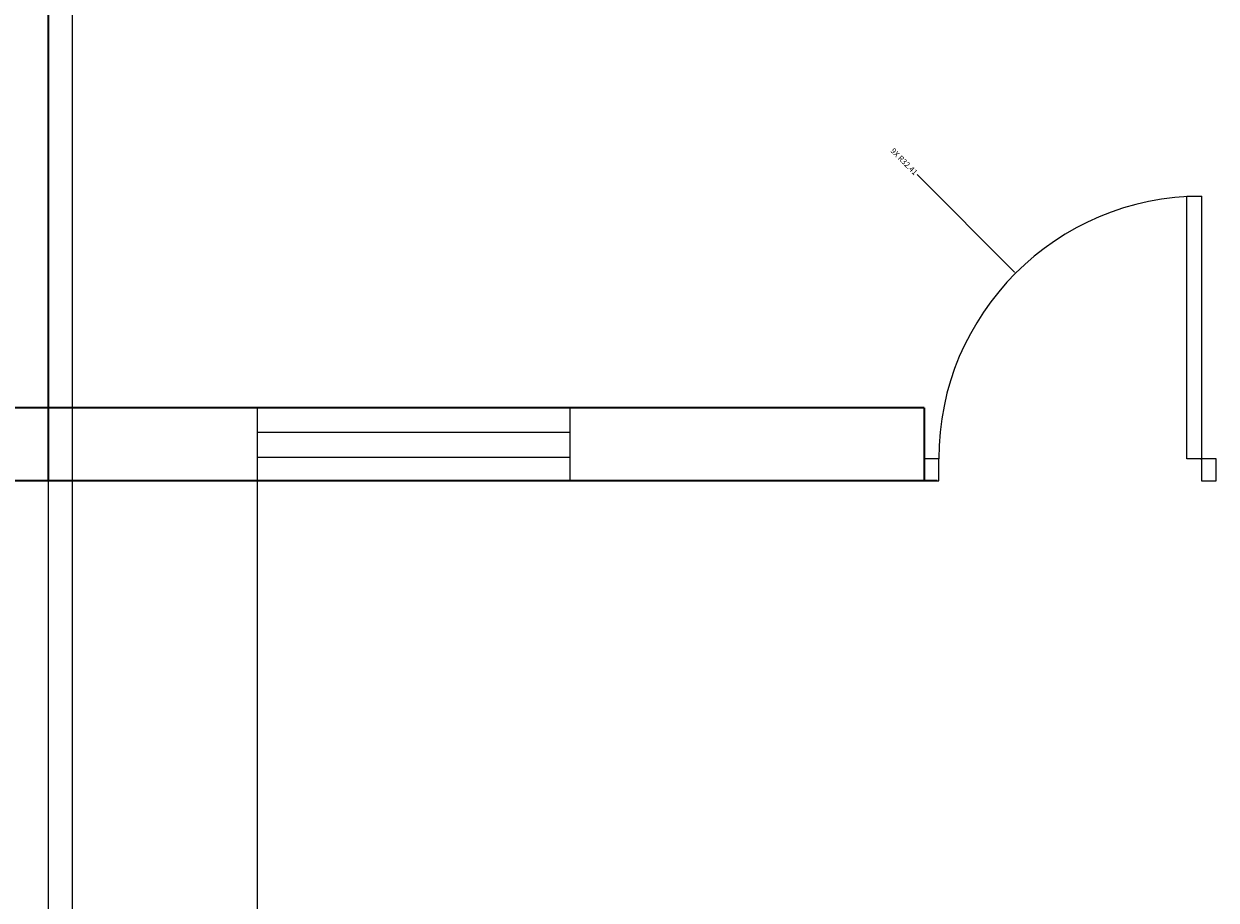
# Model space of a CAD drawing. Units: inches. Extents: x 867 to 1667, y -234 to 788.
# Tile 32 of 42: x 1074 to 1221, y 572 to 680. Entities that reach past the tile are written whole.
import ezdxf

# ---------------------------------------------------------------- set-up
doc = ezdxf.new("R2010")
doc.units = ezdxf.units.IN
doc.header["$MEASUREMENT"] = 0
for name, color, linetype, lineweight in [('A-ANNO-DIMS', 2, 'Continuous', 18), ('A-Door', 150, 'Continuous', 25), ('A-Glaz', 92, 'Continuous', 18), ('A-Wall', 7, 'Continuous', 35)]:
    doc.layers.add(name, color=color, linetype=linetype, lineweight=lineweight)
doc.layers.add('NET 01', color=8, linetype='Continuous')
doc.styles.get("Standard").update_dxf_attribs({"font": 'arial.ttf'})
doc.dimstyles.get("Standard").update_dxf_attribs({"dimtxt": 0.6875, "dimasz": 0.18, "dimexe": 0.18, "dimexo": 0.0625, "dimgap": 0.09, "dimtad": 0, "dimdec": 4, "dimzin": 0, "dimdsep": 46, "dimlunit": 4, "dimtxsty": 'Standard', "dimcen": 0.09, "dimadec": 0, "dimazin": 0, "dimtfac": 1, "dimtdec": 4, "dimtofl": 0, "dimtmove": 0, "dimatfit": 3, "dimfxl": 1, "dimtolj": 1, "dimtzin": 0, "dimarcsym": 0})

# ---------------------------------------------------------------- blocks, each defined once
blk = doc.blocks.new('A$C292B336C')
at = {"layer": 'A-Door'}
for points in [[(-0.05, 0), (-0.05, 0.9), (0, 0.9), (0, 0)], [(-0.95, 0), (-0.95, -0.075), (-0.9, -0.075), (-0.9, 0)], [(0, 0), (0, -0.075), (0.05, -0.075), (0.05, 0)]]:
    blk.add_lwpolyline(points, close=True, dxfattribs=at)
at = {"layer": 'NET 01'}
blk.add_arc((0, 0), 0.9, 90, 180, dxfattribs=at)
blk = doc.blocks.new('WIN-38_58IN')
for p, q in [((0, 9), (0, 0)), ((38.58, 0), (38.58, 9)), ((0, 6), (38.58, 6)), ((0, 2.92), (38.58, 2.92)), ((0, 0), (38.58, 0))]:
    blk.add_line(p, q)
blk = doc.blocks.new('*D29')
at = {"layer": 'A-ANNO-DIMS', "color": 0, "lineweight": -2, "transparency": 16777216}
for p, q in [((1076.89, 623.55), (1076.89, -233.54)), ((1102.67, 623.55), (1102.67, -233.54)), ((1077.07, -233.36), (1088.52, -233.36)), ((1102.49, -233.36), (1091.03, -233.36))]:
    blk.add_line(p, q, dxfattribs=at)
at = {"layer": 'A-ANNO-DIMS', "color": 0, "transparency": 16777216}
for points in [[(1077.07, -233.33), (1077.07, -233.39), (1076.89, -233.36)], [(1102.49, -233.33), (1102.49, -233.39), (1102.67, -233.36)]]:
    blk.add_solid(points, dxfattribs=at)
at = {"layer": 'Defpoints', "color": 0, "transparency": 16777216}
for p in [(1076.89, 623.62), (1102.67, 623.62), (1102.67, -233.36)]:
    blk.add_point(p, dxfattribs=at)
at = {"layer": 'A-ANNO-DIMS', "color": 0, "transparency": 16777216, "insert": (1089.78, -233.36), "char_height": 0.688, "attachment_point": 5}
blk.add_mtext('\\A1;25.78', dxfattribs=at)
blk = doc.blocks.new('*D31')
at = {"layer": 'A-ANNO-DIMS', "color": 0, "lineweight": -2, "transparency": 16777216}
for p, q in [((1070.89, 566.68), (1070.89, 787.75)), ((1071.07, 787.57), (1304.02, 787.57)), ((1538.71, 787.57), (1305.75, 787.57)), ((1538.89, 566.68), (1538.89, 787.75))]:
    blk.add_line(p, q, dxfattribs=at)
at = {"layer": 'A-ANNO-DIMS', "color": 0, "transparency": 16777216}
for points in [[(1071.07, 787.6), (1071.07, 787.54), (1070.89, 787.57)], [(1538.71, 787.6), (1538.71, 787.54), (1538.89, 787.57)]]:
    blk.add_solid(points, dxfattribs=at)
at = {"layer": 'Defpoints', "color": 0, "transparency": 16777216}
for p in [(1538.89, 787.57), (1070.89, 566.62), (1538.89, 566.62)]:
    blk.add_point(p, dxfattribs=at)
at = {"layer": 'A-ANNO-DIMS', "color": 0, "transparency": 16777216, "insert": (1304.89, 787.57), "char_height": 0.688, "attachment_point": 5}
blk.add_mtext('\\A1;468', dxfattribs=at)
blk = doc.blocks.new('*D32')
at = {"layer": 'A-ANNO-DIMS', "color": 0, "lineweight": -2, "transparency": 16777216}
for p, q in [((1079.89, 404.68), (1079.89, 787.75)), ((1080.07, 787.57), (1163.07, 787.57)), ((1247.71, 787.57), (1164.7, 787.57)), ((1247.89, 413.68), (1247.89, 787.75))]:
    blk.add_line(p, q, dxfattribs=at)
at = {"layer": 'A-ANNO-DIMS', "color": 0, "transparency": 16777216}
for points in [[(1080.07, 787.6), (1080.07, 787.54), (1079.89, 787.57)], [(1247.71, 787.6), (1247.71, 787.54), (1247.89, 787.57)]]:
    blk.add_solid(points, dxfattribs=at)
at = {"layer": 'Defpoints', "color": 0, "transparency": 16777216}
for p in [(1247.89, 787.57), (1247.89, 413.62), (1079.89, 404.62)]:
    blk.add_point(p, dxfattribs=at)
at = {"layer": 'A-ANNO-DIMS', "color": 0, "transparency": 16777216, "insert": (1163.89, 787.57), "char_height": 0.688, "attachment_point": 5}
blk.add_mtext('\\A1;168', dxfattribs=at)
blk = doc.blocks.new('*D64')
at = {"layer": 'A-ANNO-DIMS', "color": 0, "lineweight": -2, "transparency": 16777216}
for p, q in [((1184.01, 661.4), (1196.04, 649.37)), ((1219, 626.32), (1219.18, 626.32)), ((1219.09, 626.23), (1219.09, 626.41))]:
    blk.add_line(p, q, dxfattribs=at)
at = {"layer": 'A-ANNO-DIMS', "color": 0, "transparency": 16777216}
blk.add_solid([(1196.07, 649.39), (1196.02, 649.34), (1196.17, 649.24)], dxfattribs=at)
at = {"layer": 'Defpoints', "color": 0, "transparency": 16777216}
for p in [(1196.17, 649.24), (1219.09, 626.32)]:
    blk.add_point(p, dxfattribs=at)
at = {"layer": 'A-ANNO-DIMS', "color": 0, "transparency": 16777216, "insert": (1182.42, 662.99), "char_height": 0.6875, "attachment_point": 5, "rotation": 314.9925}
blk.add_mtext('\\A1;9X R32.41', dxfattribs=at)

msp = doc.modelspace()

# ---------------------------------------------------------------- linework, layer by layer
at = {"layer": 'A-Wall'}
for p, q in [((1076.8866, 740.617), (1076.8866, 623.617)), ((1184.8866, 632.617), (1067.8866, 632.617)), ((1184.8866, 632.617), (1184.8866, 623.617)), ((1186.5048, 623.617), (1067.8866, 623.617))]:
    msp.add_line(p, q, dxfattribs=at)

# ---------------------------------------------------------------- block references
at = {"layer": 'A-Door', "xscale": 36.01171521992244, "yscale": 36.01171521992244, "zscale": 36.01171521992244}
msp.add_blockref('A$C292B336C', (1219.086, 626.3179), dxfattribs=at)
at = {"layer": 'A-Glaz'}
msp.add_blockref('WIN-38_58IN', (1102.6666, 623.617), dxfattribs=at)

# ---------------------------------------------------------------- dimensions: what is measured, and where the dimension line sits
at = {"layer": 'A-ANNO-DIMS'}
for base, p1, p2, override, picture, middle in [((1538.8866, 787.567), (1070.8866, 566.617), (1538.8866, 566.617), {"dimdec": 0, "dimlfac": 1, "dimrnd": 0, "dimzin": 0, "dimdsep": 46, "dimlunit": 2}, '*D31', (1304.8866, 787.567)), ((1247.8866, 787.567), (1079.8866, 404.617), (1247.8866, 413.617), {"dimdec": 0, "dimlfac": 1, "dimrnd": 0, "dimzin": 0, "dimdsep": 46, "dimlunit": 2}, '*D32', (1163.8866, 787.567)), ((1102.6661, -233.3581), (1076.8866, 623.617), (1102.6661, 623.617), {"dimdec": 2, "dimlfac": 1, "dimrnd": 0, "dimzin": 0, "dimdsep": 46, "dimlunit": 2}, '*D29', (1089.7763, -233.3581))]:
    dim = msp.add_linear_dim(base=base, p1=p1, p2=p2, dimstyle='Standard', override=override, dxfattribs=at)
    dim.commit()
    dim.dimension.update_dxf_attribs({"geometry": picture, "text_midpoint": middle})
dim = msp.add_radius_dim(center=(1219.086, 626.3179), mpoint=(1196.1713, 649.2387), text='9X <>', dimstyle='Standard', override={"dimdec": 2, "dimlfac": 1, "dimrnd": 0, "dimzin": 0, "dimdsep": 46, "dimlunit": 2}, dxfattribs=at)
dim.commit()
dim.dimension.update_dxf_attribs({"geometry": '*D64', "text_midpoint": (1182.4225, 662.9911), "dimtype": 164})

doc.saveas('drawing.dxf')
